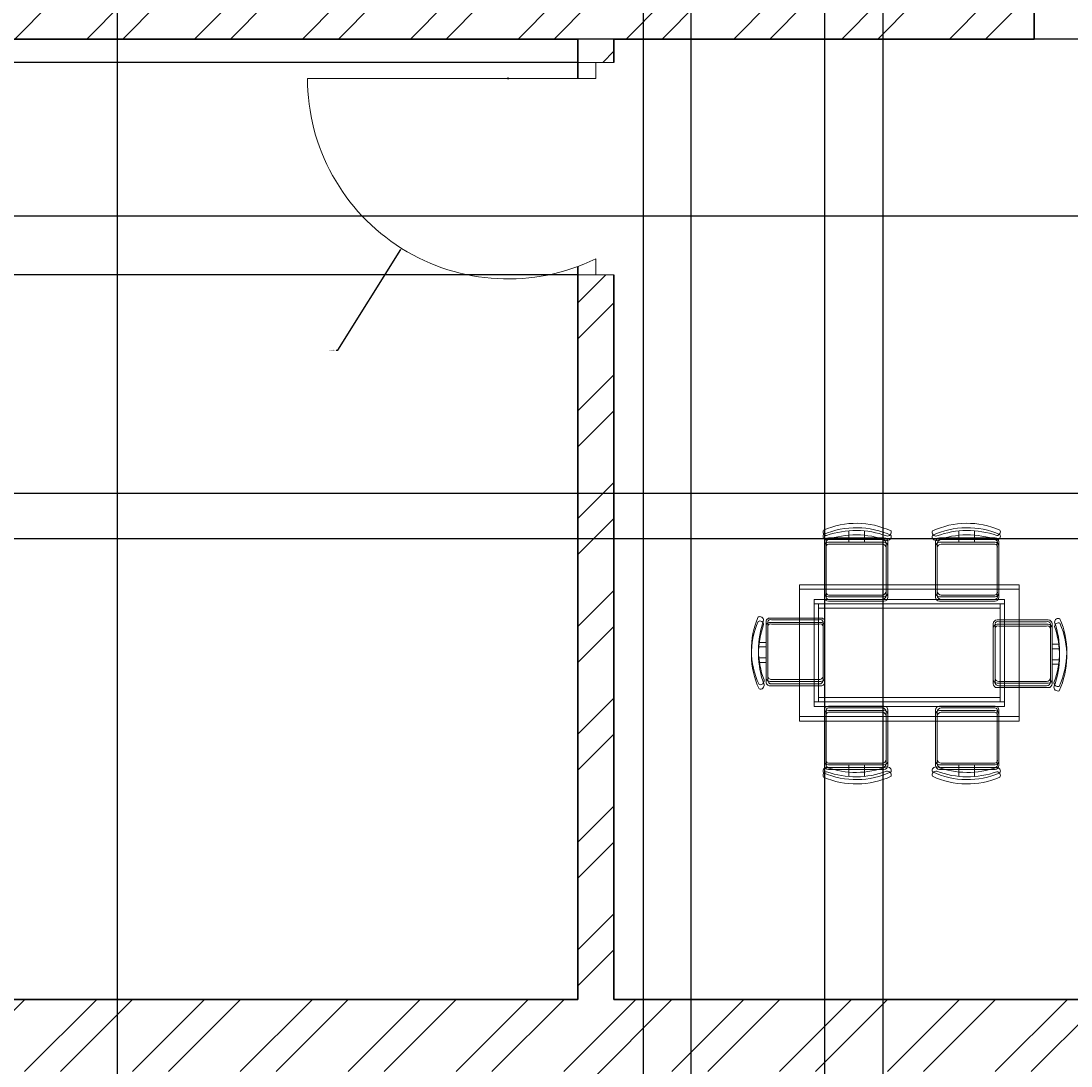
# Model space of a CAD drawing. Units: inches. Extents: x 1748 to 2382, y 1346 to 2284.
# Tile 21 of 26: x 1956 to 2088, y 1971 to 2102. Entities that reach past the tile are written whole.
import ezdxf

# ---------------------------------------------------------------- set-up
doc = ezdxf.new("R2010")
doc.units = ezdxf.units.IN
for name, color, linetype, lineweight in [('A-ANNO-DIMS', 2, 'Continuous', 18), ('A-DOOR', 21, 'Continuous', 18), ('A-FURN', 8, 'Continuous', 13), ('A-WALL', 7, 'Continuous', 35), ('A-WALL-PATT', 9, 'Continuous', 13)]:
    doc.layers.add(name, color=color, linetype=linetype, lineweight=lineweight)
doc.styles.get("Standard").update_dxf_attribs({"font": 'arial.ttf'})
doc.dimstyles.get("Standard").update_dxf_attribs({"dimtxt": 0.18, "dimasz": 0.18, "dimexe": 0.18, "dimexo": 0.0625, "dimgap": 0.09, "dimtad": 0, "dimtih": 1, "dimtoh": 1, "dimdec": 4, "dimzin": 0, "dimdsep": 46, "dimtxsty": 'Standard', "dimcen": 0.09, "dimadec": 0, "dimazin": 0, "dimtfac": 1, "dimtdec": 4, "dimtofl": 0, "dimtmove": 0, "dimatfit": 3, "dimfxl": 1, "dimtolj": 1, "dimtzin": 0, "dimarcsym": 0})

# ---------------------------------------------------------------- blocks, each defined once
blk = doc.blocks.new('TABLE-DINING')
for points in [[(0, 17.02), (27.45, 17.02), (27.45, 0.55), (0, 0.55)], [(0, 17.02), (27.45, 17.02), (27.45, 0.55), (0, 0.55)], [(0, 16.47), (27.45, 16.47), (27.45, 0), (0, 0)], [(0, 16.47), (27.45, 16.47), (27.45, 0), (0, 0)], [(1.83, 15.19), (25.62, 15.19), (25.62, 2.38), (1.83, 2.38)], [(1.83, 15.19), (25.62, 15.19), (25.62, 2.38), (1.83, 2.38)], [(1.83, 14.64), (25.62, 14.64), (25.62, 1.83), (1.83, 1.83)], [(1.83, 14.64), (25.62, 14.64), (25.62, 1.83), (1.83, 1.83)], [(2.38, 14.64), (25.07, 14.64), (25.07, 2.93), (2.38, 2.93)], [(2.38, 14.64), (25.07, 14.64), (25.07, 2.93), (2.38, 2.93)], [(2.38, 14.09), (25.07, 14.09), (25.07, 2.38), (2.38, 2.38)], [(2.38, 14.09), (25.07, 14.09), (25.07, 2.38), (2.38, 2.38)]]:
    blk.add_lwpolyline(points, close=True)
blk = doc.blocks.new('CHAIR-DINING-END')
for points in [[(7.35, 8.4, 0.414214), (6.87, 8.88), (0.49, 8.88, 0.414214), (0, 8.4), (0, 1.46, 0.414214), (0.49, 0.97), (6.87, 0.97, 0.414214), (7.35, 1.46), (7.35, 8.4)], [(7.35, 8.4, 0.414214), (6.87, 8.88), (0.49, 8.88, 0.414214), (0, 8.4), (0, 1.46, 0.414214), (0.49, 0.97), (6.87, 0.97, 0.414214), (7.35, 1.46), (7.35, 8.4)], [(7.35, 7.85, 0.414214), (6.87, 8.33), (0.49, 8.33, 0.414214), (0, 7.85), (0, 0.91, 0.414214), (0.49, 0.42), (6.87, 0.42, 0.414214), (7.35, 0.91), (7.35, 7.85)], [(7.35, 7.85, 0.414214), (6.87, 8.33), (0.49, 8.33, 0.414214), (0, 7.85), (0, 0.91, 0.414214), (0.49, 0.42), (6.87, 0.42, 0.414214), (7.35, 0.91), (7.35, 7.85)], [(7.65, 8.61, -0.175809), (7.6, 1.14, 0.578392), (8.22, 0.57, 0.214524), (8.33, 9.01, 0.552014), (7.65, 8.61, -0.065079)], [(7.65, 8.61, -0.175809), (7.6, 1.14, 0.578392), (8.22, 0.57, 0.214524), (8.33, 9.01, 0.552014), (7.65, 8.61, -0.065079)], [(7.65, 8.06, -0.175809), (7.6, 0.59, 0.578392), (8.22, 0.02, 0.214524), (8.33, 8.46, 0.552014), (7.65, 8.06, -0.065079)], [(7.65, 8.06, -0.175809), (7.6, 0.59, 0.578392), (8.22, 0.02, 0.214524), (8.33, 8.46, 0.552014), (7.65, 8.06, -0.065079)], [(7.35, 3.89), (8.23, 3.89, -0.064759)], [(7.35, 3.89), (8.23, 3.89, -0.064759)], [(7.35, 3.34), (8.23, 3.34, -0.064759)], [(7.35, 3.34), (8.23, 3.34, -0.064759)]]:
    blk.add_lwpolyline(points, format="xyb")
for points in [[(7.13, 8.39), (7.13, 1.67, -0.414214), (6.65, 1.19), (0.7, 1.19, -0.414214), (0.22, 1.67), (0.22, 8.39, -0.512069), (0.7, 8.66), (6.65, 8.66, -0.512069)], [(7.13, 8.39), (7.13, 1.67, -0.414214), (6.65, 1.19), (0.7, 1.19, -0.414214), (0.22, 1.67), (0.22, 8.39, -0.512069), (0.7, 8.66), (6.65, 8.66, -0.512069)], [(7.13, 7.84), (7.13, 1.13, -0.414214), (6.65, 0.64), (0.7, 0.64, -0.414214), (0.22, 1.13), (0.22, 7.84, -0.512069), (0.7, 8.11), (6.65, 8.11, -0.512069)], [(7.13, 7.84), (7.13, 1.12, -0.414214), (6.65, 0.64), (0.7, 0.64, -0.414214), (0.22, 1.12), (0.22, 7.84, -0.512069), (0.7, 8.11), (6.65, 8.11, -0.512069)]]:
    blk.add_lwpolyline(points, format="xyb", close=True)
for points in [[(8.25, 5.84), (7.35, 5.84)], [(8.25, 5.84), (7.35, 5.84)], [(8.25, 5.29), (7.35, 5.29)], [(8.25, 5.29), (7.35, 5.29)]]:
    blk.add_lwpolyline(points)
blk = doc.blocks.new('*D51')
at = {"layer": 'A-ANNO-DIMS', "color": 0, "lineweight": -2, "transparency": 16777216}
for p, q in [((1968.44, 2223.79), (1968.44, 1360.47)), ((2040.07, 2223.79), (2040.07, 1360.47)), ((1968.62, 1360.65), (2003.86, 1360.65)), ((2039.89, 1360.65), (2004.65, 1360.65))]:
    blk.add_line(p, q, dxfattribs=at)
at = {"layer": 'A-ANNO-DIMS', "color": 0, "transparency": 16777216}
for points in [[(1968.62, 1360.68), (1968.62, 1360.62), (1968.44, 1360.65)], [(2039.89, 1360.68), (2039.89, 1360.62), (2040.07, 1360.65)]]:
    blk.add_solid(points, dxfattribs=at)
at = {"layer": 'Defpoints', "color": 0, "transparency": 16777216}
for p in [(1968.44, 2223.85), (2040.07, 2223.85), (2040.07, 1360.65)]:
    blk.add_point(p, dxfattribs=at)
at = {"layer": 'A-ANNO-DIMS', "color": 0, "transparency": 16777216, "insert": (2004.26, 1360.65), "char_height": 0.18, "attachment_point": 5}
blk.add_mtext('\\A1;71.62', dxfattribs=at)
blk = doc.blocks.new('*D52')
at = {"layer": 'A-ANNO-DIMS', "color": 0, "lineweight": -2, "transparency": 16777216}
for p, q in [((2064.07, 2223.79), (2064.07, 1360.47)), ((2091.4, 2223.79), (2091.4, 1360.47)), ((2064.25, 1360.65), (2077.34, 1360.65)), ((2091.22, 1360.65), (2078.13, 1360.65))]:
    blk.add_line(p, q, dxfattribs=at)
at = {"layer": 'A-ANNO-DIMS', "color": 0, "transparency": 16777216}
for points in [[(2064.25, 1360.68), (2064.25, 1360.62), (2064.07, 1360.65)], [(2091.22, 1360.68), (2091.22, 1360.62), (2091.4, 1360.65)]]:
    blk.add_solid(points, dxfattribs=at)
at = {"layer": 'Defpoints', "color": 0, "transparency": 16777216}
for p in [(2064.07, 2223.85), (2091.4, 2223.85), (2091.4, 1360.65)]:
    blk.add_point(p, dxfattribs=at)
at = {"layer": 'A-ANNO-DIMS', "color": 0, "transparency": 16777216, "insert": (2077.73, 1360.65), "char_height": 0.18, "attachment_point": 5}
blk.add_mtext('\\A1;27.33', dxfattribs=at)
blk = doc.blocks.new('*D57')
at = {"layer": 'A-ANNO-DIMS', "color": 0, "lineweight": -2, "transparency": 16777216}
for p, q in [((2288.4, 2099.35), (1779.88, 2099.35)), ((1780.06, 2099.17), (1780.06, 2088.46)), ((1780.06, 2077.38), (1780.06, 2088.09)), ((2288.4, 2077.2), (1779.88, 2077.2))]:
    blk.add_line(p, q, dxfattribs=at)
at = {"layer": 'A-ANNO-DIMS', "color": 0, "transparency": 16777216}
for points in [[(1780.03, 2099.17), (1780.09, 2099.17), (1780.06, 2099.35)], [(1780.03, 2077.38), (1780.09, 2077.38), (1780.06, 2077.2)]]:
    blk.add_solid(points, dxfattribs=at)
at = {"layer": 'Defpoints', "color": 0, "transparency": 16777216}
for p in [(1780.06, 2099.35), (2288.46, 2099.35), (2288.46, 2077.2)]:
    blk.add_point(p, dxfattribs=at)
at = {"layer": 'A-ANNO-DIMS', "color": 0, "transparency": 16777216, "insert": (1780.06, 2088.28), "char_height": 0.18, "attachment_point": 5}
blk.add_mtext('\\A1;22.15', dxfattribs=at)
blk = doc.blocks.new('*D63')
at = {"layer": 'A-ANNO-DIMS', "color": 0, "lineweight": -2, "transparency": 16777216}
for p, q in [((2253.72, 2042.57), (1779.88, 2042.57)), ((1780.06, 2042.39), (1780.06, 2039.92)), ((1780.06, 2037.08), (1780.06, 2039.55)), ((2253.72, 2036.9), (1779.88, 2036.9))]:
    blk.add_line(p, q, dxfattribs=at)
at = {"layer": 'A-ANNO-DIMS', "color": 0, "transparency": 16777216}
for points in [[(1780.03, 2042.39), (1780.09, 2042.39), (1780.06, 2042.57)], [(1780.03, 2037.08), (1780.09, 2037.08), (1780.06, 2036.9)]]:
    blk.add_solid(points, dxfattribs=at)
at = {"layer": 'Defpoints', "color": 0, "transparency": 16777216}
for p in [(1780.06, 2042.57), (2253.78, 2042.57), (2253.78, 2036.9)]:
    blk.add_point(p, dxfattribs=at)
at = {"layer": 'A-ANNO-DIMS', "color": 0, "transparency": 16777216, "insert": (1780.06, 2039.74), "char_height": 0.18, "attachment_point": 5}
blk.add_mtext('\\A1;5.673', dxfattribs=at)
blk = doc.blocks.new('*D76')
at = {"layer": 'A-ANNO-DIMS', "color": 0, "lineweight": -2, "transparency": 16777216}
for p, q in [((2025.9, 2096.43), (1779.88, 2096.43)), ((1780.06, 2096.25), (1780.06, 2083.35)), ((1780.06, 2070.08), (1780.06, 2082.98)), ((2025.9, 2069.9), (1779.88, 2069.9))]:
    blk.add_line(p, q, dxfattribs=at)
at = {"layer": 'A-ANNO-DIMS', "color": 0, "transparency": 16777216}
for points in [[(1780.03, 2096.25), (1780.09, 2096.25), (1780.06, 2096.43)], [(1780.03, 2070.08), (1780.09, 2070.08), (1780.06, 2069.9)]]:
    blk.add_solid(points, dxfattribs=at)
at = {"layer": 'Defpoints', "color": 0, "transparency": 16777216}
for p in [(1780.06, 2096.43), (2025.96, 2096.43), (2025.96, 2069.9)]:
    blk.add_point(p, dxfattribs=at)
at = {"layer": 'A-ANNO-DIMS', "color": 0, "transparency": 16777216, "insert": (1780.06, 2083.16), "char_height": 0.18, "attachment_point": 5}
blk.add_mtext('\\A1;26.535', dxfattribs=at)
blk = doc.blocks.new('*D78')
at = {"layer": 'A-ANNO-DIMS', "color": 0, "lineweight": -2, "transparency": 16777216}
for p, q in [((2034.13, 2132.54), (2034.13, 1360.47)), ((2056.8, 2127.06), (2056.8, 1360.47)), ((2034.31, 1360.65), (2045, 1360.65)), ((2056.62, 1360.65), (2045.93, 1360.65))]:
    blk.add_line(p, q, dxfattribs=at)
at = {"layer": 'A-ANNO-DIMS', "color": 0, "transparency": 16777216}
for points in [[(2034.31, 1360.68), (2034.31, 1360.62), (2034.13, 1360.65)], [(2056.62, 1360.68), (2056.62, 1360.62), (2056.8, 1360.65)]]:
    blk.add_solid(points, dxfattribs=at)
at = {"layer": 'Defpoints', "color": 0, "transparency": 16777216}
for p in [(2034.13, 2132.6), (2056.8, 2127.13), (2056.8, 1360.65)]:
    blk.add_point(p, dxfattribs=at)
at = {"layer": 'A-ANNO-DIMS', "color": 0, "transparency": 16777216, "insert": (2045.47, 1360.65), "char_height": 0.18, "attachment_point": 5}
blk.add_mtext('\\A1;22.663', dxfattribs=at)
blk = doc.blocks.new('*D87')
at = {"layer": 'A-ANNO-DIMS', "color": 0, "lineweight": -2, "transparency": 16777216}
for p, q in [((2017.17, 2094.43), (2017.35, 2094.43)), ((2017.26, 2094.34), (2017.26, 2094.52)), ((1995.99, 2060.46), (2003.88, 2073.04)), ((1995.81, 2060.46), (1995.99, 2060.46))]:
    blk.add_line(p, q, dxfattribs=at)
at = {"layer": 'A-ANNO-DIMS', "color": 0, "transparency": 16777216}
blk.add_solid([(2003.85, 2073.06), (2003.9, 2073.03), (2003.97, 2073.2)], dxfattribs=at)
at = {"layer": 'Defpoints', "color": 0, "transparency": 16777216}
for p in [(2017.26, 2094.43), (2003.97, 2073.2)]:
    blk.add_point(p, dxfattribs=at)
at = {"layer": 'A-ANNO-DIMS', "color": 0, "transparency": 16777216, "insert": (1995.27, 2060.46), "char_height": 0.18, "attachment_point": 5}
blk.add_mtext('\\A1;R25.053', dxfattribs=at)

msp = doc.modelspace()

# ---------------------------------------------------------------- hatches: boundary and pattern name
at = {"layer": 'A-WALL-PATT'}
h = msp.add_hatch(dxfattribs=at)
h.set_pattern_fill('ANSI32', color=256)
h.paths.add_polyline_path([(1908.4445, 2232.8497), (1821.9607, 2232.8497), (1821.9607, 2223.8497), (1865.4607, 2223.8497), (1865.4607, 2209.9185), (1869.9607, 2209.9185), (1869.9607, 2223.8497), (1908.4445, 2223.8497), (1908.4445, 2228.3497)])
h.paths.add_polyline_path([(2040.0683, 2232.8497), (1968.4445, 2232.8497), (1968.4445, 2223.8497), (2025.9607, 2223.8497), (2025.9607, 2130.3497), (2032.1341, 2130.3497), (2032.1341, 2132.5997), (2032.1341, 2134.8497), (2030.4607, 2134.8497), (2030.4607, 2223.8497), (2040.0683, 2223.8497)])
h.paths.add_polyline_path([(2091.3969, 2232.8497), (2064.0683, 2232.8497), (2064.0683, 2223.8497), (2078.4607, 2223.8497), (2078.4607, 2134.8497), (2051.1563, 2134.8497), (2051.1563, 2130.3497), (2078.4607, 2130.3497), (2078.4607, 2128.6813), (2082.9607, 2128.6813), (2082.9607, 2130.3497), (2086.1879, 2130.3497), (2086.1879, 2132.5997), (2086.1879, 2134.8497), (2082.9607, 2134.8497), (2082.9607, 2223.8497), (2091.3969, 2223.8497), (2091.3969, 2228.3497)])
h.paths.add_polyline_path([(2167.0164, 2232.8497), (2115.3969, 2232.8497), (2115.3969, 2223.8497), (2130.9607, 2223.8497), (2130.9607, 2134.8497), (2106.9607, 2134.8497), (2106.9607, 2130.3497), (2135.4607, 2130.3497), (2135.4607, 2223.8497), (2167.0164, 2223.8497), (2167.0164, 2228.3497)])
h.paths.add_polyline_path([(1869.9607, 2149.9185), (1865.4607, 2149.9185), (1865.4607, 2127.8942), (1869.9607, 2127.8942)])
h.paths.add_polyline_path([(2082.9607, 2104.4871), (2080.7107, 2104.4871), (2078.4607, 2104.4871), (2078.4607, 2103.8497), (1869.9607, 2103.8497), (1869.9607, 2108.6062), (1867.7107, 2108.6062), (1865.4607, 2108.6062), (1865.4607, 2103.8497), (1821.9607, 2103.8497), (1821.9607, 2099.3497), (1865.4607, 2099.3497), (1865.4607, 2094.7509), (1869.9607, 2094.7509), (1869.9607, 2099.3497), (2025.9607, 2099.3497), (2025.9607, 2096.4326), (2030.4607, 2096.4326), (2030.4607, 2099.3497), (2082.9607, 2099.3497)])
h.paths.add_polyline_path([(1928.9457, 1401.1212), (2176.8693, 1401.1212), (2176.8693, 1438.214), (1928.9457, 1438.214)], flags=9)
h.paths.add_polyline_path([(2122.2668, 2048.1927), (2177.9387, 2048.1927), (2177.9387, 2066.85), (2122.2668, 2066.85)], flags=9)
h.paths.add_polyline_path([(2272.688, 2153.8197), (2272.688, 2216.746), (2262.3845, 2216.746), (2262.3845, 2153.8197)], flags=9)
h.paths.add_polyline_path([(2157.2928, 2166.5593), (2196.3822, 2166.5593), (2196.3822, 2185.2167), (2157.2928, 2185.2167)], flags=9)
h.paths.add_polyline_path([(2089.3407, 2162.0698), (2124.3987, 2162.0698), (2124.3987, 2180.7272), (2089.3407, 2180.7272)], flags=9)
h.paths.add_polyline_path([(2037.4521, 2160.0913), (2072.5101, 2160.0913), (2072.5101, 2178.7486), (2037.4521, 2178.7486)], flags=9)
h.paths.add_polyline_path([(1884.7894, 2104.1554), (1923.6297, 2104.1554), (1923.6297, 2122.8127), (1884.7894, 2122.8127)], flags=9)
h.paths.add_polyline_path([(1851.2832, 2142.9749), (1851.2832, 2199.3051), (1840.9796, 2199.3051), (1840.9796, 2142.9749)], flags=9)
h.paths.add_polyline_path([(1844.8763, 2017.2834), (1844.8763, 2073.6136), (1834.5728, 2073.6136), (1834.5728, 2017.2834)], flags=9)
h.paths.add_polyline_path([(1897.1577, 2073.1279), (1935.9981, 2073.1279), (1935.9981, 2091.7853), (1897.1577, 2091.7853)], flags=9)
h.paths.add_polyline_path([(1952.3395, 1802.4231), (2008.0114, 1802.4231), (2008.0114, 1821.0805), (1952.3395, 1821.0805)], flags=9)
h.paths.add_polyline_path([(1978.8184, 1857.6841), (2017.7338, 1857.6841), (2017.7338, 1876.3415), (1978.8184, 1876.3415)], flags=9)
h.paths.add_polyline_path([(1979.6513, 1925.9516), (2008.8089, 1925.9516), (2008.8089, 1944.6089), (1979.6513, 1944.6089)], flags=9)
h.paths.add_polyline_path([(1838.5553, 1860.3527), (1877.3957, 1860.3527), (1877.3957, 1879.01), (1838.5553, 1879.01)], flags=9)
h.paths.add_polyline_path([(1883.9018, 1787.3013), (1883.9018, 1843.6315), (1873.5983, 1843.6315), (1873.5983, 1787.3013)], flags=9)
h.paths.add_polyline_path([(1873.7079, 1509.1938), (1873.7079, 1583.7709), (1863.4044, 1583.7709), (1863.4044, 1509.1938)], flags=9)
h.paths.add_polyline_path([(1916.2259, 1603.3681), (1955.0663, 1603.3681), (1955.0663, 1622.0254), (1916.2259, 1622.0254)], flags=9)
h.paths.add_polyline_path([(1876.3013, 1636.757), (1876.3013, 1693.0871), (1865.9978, 1693.0871), (1865.9978, 1636.757)], flags=9)
h.paths.add_polyline_path([(1921.3138, 1521.8316), (1964.0662, 1521.8316), (1964.0662, 1540.489), (1921.3138, 1540.489)], flags=9)
h.paths.add_polyline_path([(2017.5657, 1497.5078), (2046.7983, 1497.5078), (2046.7983, 1516.1651), (2017.5657, 1516.1651)], flags=9)
h.paths.add_polyline_path([(2066.8661, 1499.3902), (2096.0988, 1499.3902), (2096.0988, 1518.0475), (2066.8661, 1518.0475)], flags=9)
h.paths.add_polyline_path([(2155.4835, 1571.6596), (2198.2358, 1571.6596), (2198.2358, 1590.3169), (2155.4835, 1590.3169)], flags=9)
h.paths.add_polyline_path([(2094.9136, 1664.6812), (2150.5855, 1664.6812), (2150.5855, 1683.3386), (2094.9136, 1683.3386)], flags=9)
h.paths.add_polyline_path([(2257.6902, 1863.1628), (2269.8935, 1863.1628), (2269.8935, 1873.4664), (2257.6902, 1873.4664)], flags=9)
h.paths.add_polyline_path([(2164.0748, 1880.3089), (2189.8694, 1880.3089), (2189.8694, 1890.6124), (2164.0748, 1890.6124)], flags=9)
h.paths.add_polyline_path([(2239.4394, 1931.0585), (2268.8187, 1931.0585), (2268.8187, 1949.7159), (2239.4394, 1949.7159)], flags=9)
h = msp.add_hatch(dxfattribs=at)
h.set_pattern_fill('ANSI32', color=256)
h.paths.add_polyline_path([(1900.6426, 1652.723), (1896.1426, 1652.723), (1896.1426, 1629.9029), (1900.6426, 1629.9029)])
h.paths.add_polyline_path([(2206.0699, 1859.3497), (2197.0699, 1859.3497), (2197.0699, 1734.8497), (2206.0699, 1734.8497)], flags=17)
h.paths.add_polyline_path([(2297.4607, 1865.3269), (2288.4607, 1865.3269), (2288.4607, 1734.8497), (2206.0699, 1734.8497), (2180.4551, 1734.8497), (2180.4551, 1725.8497), (2197.0699, 1725.8497), (2206.0699, 1725.8497), (2288.4607, 1725.8497), (2288.4607, 1705.3038), (2297.4607, 1705.3038)])
h.paths.add_polyline_path([(2139.9607, 1815.8001), (2135.4607, 1815.8001), (2130.9607, 1815.8001), (2130.9607, 1734.8497), (1900.6426, 1734.8497), (1900.6426, 1738.9477), (1898.3926, 1738.9477), (1896.1426, 1738.9477), (1896.1426, 1734.8497), (1857.1426, 1734.8497), (1857.1426, 1725.8497), (1896.1426, 1725.8497), (1896.1426, 1712.723), (1900.6426, 1712.723), (1900.6426, 1725.8497), (2006.4607, 1725.8497), (2006.4607, 1637.448), (2010.9607, 1637.448), (2010.9607, 1725.8497), (2139.9607, 1725.8497), (2147.389, 1725.8497), (2147.389, 1730.3497), (2147.389, 1734.8497), (2139.9607, 1734.8497)])
h.paths.add_polyline_path([(2149.8497, 1917.8497), (2149.8497, 1922.3497), (2139.9607, 1922.3497), (2139.9607, 1979.3497), (2030.4607, 1979.3497), (2030.4607, 2069.8971), (2028.2107, 2069.8971), (2025.9607, 2069.8971), (2025.9607, 1979.3497), (1869.9607, 1979.3497), (1869.9607, 1998.93), (1865.4607, 1998.93), (1865.4607, 1979.3497), (1821.9607, 1979.3497), (1821.9607, 1952.7922), (1826.9306, 1952.7922), (1830.9607, 1952.7922), (1830.9607, 1970.3497), (1962.9607, 1970.3497), (1962.9607, 1926.5713), (1967.4607, 1926.5713), (1967.4607, 1970.3497), (2027.4607, 1970.3497), (2027.4607, 1898.3497), (2004.9604, 1898.3497), (2004.9604, 1893.8497), (2027.4607, 1893.8497), (2027.4607, 1859.3497), (1958.8973, 1859.3497), (1958.8973, 1854.8497), (2047.917, 1854.8497), (2047.917, 1859.3497), (2031.9607, 1859.3497), (2031.9607, 1970.3497), (2130.9607, 1970.3497), (2130.9607, 1859.3497), (2104.9565, 1859.3497), (2104.9565, 1854.8497), (2130.9607, 1854.8497), (2130.9607, 1849.0684), (2139.9607, 1849.0684), (2139.9607, 1913.3497), (2149.8497, 1913.3497)])
h.paths.add_polyline_path([(1928.9996, 1859.3497), (1830.9607, 1859.3497), (1830.9607, 1892.7922), (1821.9607, 1892.7922), (1821.9607, 1854.8497), (1896.1426, 1854.8497), (1896.1426, 1836.6443), (1898.378, 1836.6443), (1900.6426, 1836.6443), (1900.6426, 1854.8497), (1928.9996, 1854.8497), (1928.9996, 1857.0997)])
h.paths.add_polyline_path([(1980.9604, 1896.0997), (1980.9604, 1898.3497), (1967.4607, 1898.3497), (1967.4607, 1902.3846), (1962.9607, 1902.3846), (1962.9607, 1859.3497), (1967.4607, 1859.3497), (1967.4607, 1893.8497), (1980.9604, 1893.8497)], flags=17)
h.paths.add_polyline_path([(1900.6426, 1776.6443), (1896.1426, 1776.6443), (1896.1426, 1758.0891), (1900.6426, 1758.0891)], flags=17)
h.paths.add_polyline_path([(2297.4607, 2017.2008), (2288.4607, 2017.2008), (2288.4607, 1979.3497), (2213.4607, 1979.3497), (2213.4607, 1922.3497), (2183.3516, 1922.3497), (2183.3516, 1913.3497), (2213.4607, 1913.3497), (2236.234, 1913.3497), (2236.234, 1922.3497), (2222.4607, 1922.3497), (2222.4607, 1931.3497), (2222.4607, 1970.3497), (2288.4607, 1970.3497), (2288.4607, 1922.3497), (2272.1921, 1922.3497), (2272.1921, 1913.3497), (2288.4607, 1913.3497), (2288.4607, 1901.3269), (2297.4607, 1901.3269)])

# ---------------------------------------------------------------- linework, layer by layer
at = {"layer": 'A-DOOR'}
for p, q in [((2025.9607, 2096.4326), (2030.4607, 2096.4326)), ((2030.4607, 2096.4326), (2028.2107, 2096.4326)), ((2028.2107, 2096.4326), (2028.2107, 2094.4326)), ((2028.2107, 2094.4326), (1992.2107, 2094.4326)), ((2028.2107, 2069.8971), (2028.2107, 2071.8971)), ((2025.9607, 2069.8971), (2030.4607, 2069.8971)), ((2030.4607, 2069.8971), (2028.2107, 2069.8971))]:
    msp.add_line(p, q, dxfattribs=at)
msp.add_arc((2017.2641, 2094.4326), 25.0534, 180, 295.908118, dxfattribs=at)
at = {"layer": 'A-FURN'}
for points in [[(2057.0522, 2037.3215, -0.17580919), (2064.5276, 2037.2649, 0.57839206), (2065.0939, 2037.8876, 0.21452438), (2056.6557, 2038.0008, 0.55201397), (2057.0522, 2037.3215, -0.06507904)], [(2057.0522, 2037.3212, -0.17580919), (2064.5276, 2037.2646, 0.57839206), (2065.0939, 2037.8873, 0.21452438), (2056.6558, 2038.0005, 0.55201397), (2057.0522, 2037.3212, -0.06507904)], [(2057.0522, 2036.7726, -0.17580919), (2064.5276, 2036.716, 0.57839206), (2065.0939, 2037.3387, 0.21452438), (2056.6557, 2037.4519, 0.55201397), (2057.0522, 2036.7726, -0.06507904)], [(2057.0522, 2036.7723, -0.17580919), (2064.5276, 2036.7157, 0.57839206), (2065.0939, 2037.3384, 0.21452438), (2056.6558, 2037.4516, 0.55201397), (2057.0522, 2036.7723, -0.06507904)], [(2070.821, 2037.2649, -0.57839206), (2070.2546, 2037.8876, -0.21452438), (2078.6928, 2038.0008, -0.55201397), (2078.2964, 2037.3215, 0.1758092), (2070.821, 2037.2649)], [(2070.821, 2037.2646, -0.57839206), (2070.2547, 2037.8873, -0.21452438), (2078.6928, 2038.0005, -0.55201397), (2078.2964, 2037.3212, 0.1758092), (2070.821, 2037.2646)], [(2070.821, 2036.716, -0.57839206), (2070.2546, 2037.3387, -0.21452438), (2078.6928, 2037.4519, -0.55201397), (2078.2964, 2036.7726, 0.1758092), (2070.821, 2036.716)], [(2070.821, 2036.7157, -0.57839206), (2070.2547, 2037.3384, -0.21452438), (2078.6928, 2037.4516, -0.55201397), (2078.2964, 2036.7723, 0.1758092), (2070.821, 2036.7157)], [(2064.2105, 2037.0215), (2057.2705, 2037.0215, 0.41421356), (2056.785, 2036.536), (2056.785, 2030.1548, 0.41421356), (2057.2705, 2029.6693), (2064.2105, 2029.6693, 0.41421356), (2064.696, 2030.1548), (2064.696, 2036.536, 0.41421356), (2064.2105, 2037.0215)], [(2064.2105, 2037.0212), (2057.2705, 2037.0212, 0.41421356), (2056.785, 2036.5357), (2056.785, 2030.1545, 0.41421356), (2057.2705, 2029.669), (2064.2105, 2029.669, 0.41421356), (2064.696, 2030.1545), (2064.696, 2036.5357, 0.41421356), (2064.2105, 2037.0212)], [(2061.7728, 2037.0215), (2061.7728, 2037.8992, -0.06475861)], [(2061.7728, 2037.0212), (2061.7728, 2037.8989, -0.06475861)], [(2061.7728, 2036.4726), (2061.7728, 2037.3503, -0.06475861)], [(2061.7728, 2036.4723), (2061.7728, 2037.35, -0.06475861)], [(2078.0781, 2037.0215, -0.41421356), (2078.5636, 2036.536), (2078.5636, 2030.1548, -0.41421356), (2078.0781, 2029.6693), (2071.1381, 2029.6693, -0.41421356), (2070.6526, 2030.1548), (2070.6526, 2036.536, -0.41421356), (2071.1381, 2037.0215), (2078.0781, 2037.0215)], [(2078.0781, 2037.0212, -0.41421356), (2078.5636, 2036.5357), (2078.5636, 2030.1545, -0.41421356), (2078.0781, 2029.669), (2071.1381, 2029.669, -0.41421356), (2070.6526, 2030.1545), (2070.6526, 2036.5357, -0.41421356), (2071.1381, 2037.0212), (2078.0781, 2037.0212)], [(2073.5758, 2037.0215), (2073.5758, 2037.8992, 0.06475861)], [(2073.5758, 2037.0212), (2073.5758, 2037.8989, 0.06475861)], [(2073.5758, 2036.4726), (2073.5758, 2037.3503, 0.06475861)], [(2073.5758, 2036.4723), (2073.5758, 2037.35, 0.06475861)], [(2064.2105, 2036.4726), (2057.2705, 2036.4726, 0.41421356), (2056.785, 2035.987), (2056.785, 2029.6059, 0.41421356), (2057.2705, 2029.1204), (2064.2105, 2029.1204, 0.41421356), (2064.696, 2029.6059), (2064.696, 2035.987, 0.41421356), (2064.2105, 2036.4726)], [(2064.2105, 2036.4723), (2057.2705, 2036.4723, 0.41421356), (2056.785, 2035.9868), (2056.785, 2029.6056, 0.41421356), (2057.2705, 2029.1201), (2064.2105, 2029.1201, 0.41421356), (2064.696, 2029.6056), (2064.696, 2035.9868, 0.41421356), (2064.2105, 2036.4723)], [(2078.0781, 2036.4726, -0.41421356), (2078.5636, 2035.987), (2078.5636, 2029.6059, -0.41421356), (2078.0781, 2029.1204), (2071.1381, 2029.1204, -0.41421356), (2070.6526, 2029.6059), (2070.6526, 2035.987, -0.41421356), (2071.1381, 2036.4726), (2078.0781, 2036.4726)], [(2078.0781, 2036.4723, -0.41421356), (2078.5636, 2035.9868), (2078.5636, 2029.6056, -0.41421356), (2078.0781, 2029.1201), (2071.1381, 2029.1201, -0.41421356), (2070.6526, 2029.6056), (2070.6526, 2035.9868, -0.41421356), (2071.1381, 2036.4723), (2078.0781, 2036.4723)], [(2085.2123, 2026.2889, 0.41421356), (2084.7268, 2026.7744), (2078.3456, 2026.7744, 0.41421356), (2077.8601, 2026.2889), (2077.8601, 2019.3489, 0.41421356), (2078.3456, 2018.8634), (2084.7268, 2018.8634, 0.41421356), (2085.2123, 2019.3489), (2085.2123, 2026.2889)], [(2085.2123, 2026.2886, 0.41421356), (2084.7268, 2026.7741), (2078.3456, 2026.7741, 0.41421356), (2077.8601, 2026.2886), (2077.8601, 2019.3486, 0.41421356), (2078.3456, 2018.8631), (2084.7268, 2018.8631, 0.41421356), (2085.2123, 2019.3486), (2085.2123, 2026.2886)], [(2085.2123, 2025.74, 0.41421356), (2084.7268, 2026.2255), (2078.3456, 2026.2255, 0.41421356), (2077.8601, 2025.74), (2077.8601, 2018.8, 0.41421356), (2078.3456, 2018.3145), (2084.7268, 2018.3145, 0.41421356), (2085.2123, 2018.8), (2085.2123, 2025.74)], [(2085.2123, 2025.7397, 0.41421356), (2084.7268, 2026.2252), (2078.3456, 2026.2252, 0.41421356), (2077.8601, 2025.7397), (2077.8601, 2018.7997, 0.41421356), (2078.3456, 2018.3142), (2084.7268, 2018.3142, 0.41421356), (2085.2123, 2018.7997), (2085.2123, 2025.7397)], [(2085.5123, 2026.5072, -0.17580919), (2085.4557, 2019.0318, 0.57839206), (2086.0784, 2018.4655, 0.21452438), (2086.1917, 2026.9036, 0.55201397), (2085.5123, 2026.5072, -0.06507904)], [(2085.5123, 2025.9583, -0.17580919), (2085.4557, 2018.4829, 0.57839206), (2086.0784, 2017.9165, 0.21452438), (2086.1917, 2026.3547, 0.55201397), (2085.5123, 2025.9583, -0.06507904)], [(2085.5123, 2026.5069, -0.17580919), (2085.4557, 2019.0315, 0.57839206), (2086.0785, 2018.4652, 0.21452438), (2086.1917, 2026.9034, 0.55201397), (2085.5123, 2026.5069, -0.06507904)], [(2085.5123, 2025.958, -0.17580919), (2085.4557, 2018.4826, 0.57839206), (2086.0785, 2017.9163, 0.21452438), (2086.1917, 2026.3544, 0.55201397), (2085.5123, 2025.958, -0.06507904)], [(2085.2123, 2021.7866), (2086.09, 2021.7866, -0.06475861)], [(2085.2123, 2021.7863), (2086.09, 2021.7863, -0.06475861)], [(2085.2123, 2021.2377), (2086.09, 2021.2377, -0.06475861)], [(2085.2123, 2021.2374), (2086.09, 2021.2374, -0.06475861)], [(2064.2105, 2008.6557), (2057.2705, 2008.6557, -0.41421356), (2056.785, 2009.1413), (2056.785, 2015.5224, -0.41421356), (2057.2705, 2016.0079), (2064.2105, 2016.0079, -0.41421356), (2064.696, 2015.5224), (2064.696, 2009.1413, -0.41421356), (2064.2105, 2008.6557)], [(2064.2105, 2008.6554), (2057.2705, 2008.6554, -0.41421356), (2056.785, 2009.141), (2056.785, 2015.5221, -0.41421356), (2057.2705, 2016.0076), (2064.2105, 2016.0076, -0.41421356), (2064.696, 2015.5221), (2064.696, 2009.141, -0.41421356), (2064.2105, 2008.6554)], [(2078.0781, 2008.6557, 0.41421356), (2078.5636, 2009.1413), (2078.5636, 2015.5224, 0.41421356), (2078.0781, 2016.0079), (2071.1381, 2016.0079, 0.41421356), (2070.6526, 2015.5224), (2070.6526, 2009.1413, 0.41421356), (2071.1381, 2008.6557), (2078.0781, 2008.6557)], [(2078.0781, 2008.6554, 0.41421356), (2078.5636, 2009.141), (2078.5636, 2015.5221, 0.41421356), (2078.0781, 2016.0076), (2071.1381, 2016.0076, 0.41421356), (2070.6526, 2015.5221), (2070.6526, 2009.141, 0.41421356), (2071.1381, 2008.6554), (2078.0781, 2008.6554)], [(2064.2105, 2008.1068), (2057.2705, 2008.1068, -0.41421356), (2056.785, 2008.5923), (2056.785, 2014.9735, -0.41421356), (2057.2705, 2015.459), (2064.2105, 2015.459, -0.41421356), (2064.696, 2014.9735), (2064.696, 2008.5923, -0.41421356), (2064.2105, 2008.1068)], [(2064.2105, 2008.1065), (2057.2705, 2008.1065, -0.41421356), (2056.785, 2008.5921), (2056.785, 2014.9732, -0.41421356), (2057.2705, 2015.4587), (2064.2105, 2015.4587, -0.41421356), (2064.696, 2014.9732), (2064.696, 2008.5921, -0.41421356), (2064.2105, 2008.1065)], [(2078.0781, 2008.1068, 0.41421356), (2078.5636, 2008.5923), (2078.5636, 2014.9735, 0.41421356), (2078.0781, 2015.459), (2071.1381, 2015.459, 0.41421356), (2070.6526, 2014.9735), (2070.6526, 2008.5923, 0.41421356), (2071.1381, 2008.1068), (2078.0781, 2008.1068)], [(2078.0781, 2008.1065, 0.41421356), (2078.5636, 2008.5921), (2078.5636, 2014.9732, 0.41421356), (2078.0781, 2015.4587), (2071.1381, 2015.4587, 0.41421356), (2070.6526, 2014.9732), (2070.6526, 2008.5921, 0.41421356), (2071.1381, 2008.1065), (2078.0781, 2008.1065)], [(2064.5276, 2008.4123, -0.57839206), (2065.0939, 2007.7896, -0.21452438), (2056.6557, 2007.6764, -0.55201397), (2057.0522, 2008.3557, 0.17580929), (2064.5276, 2008.4123)], [(2064.5276, 2008.412, -0.57839206), (2065.0939, 2007.7893, -0.21452438), (2056.6558, 2007.6761, -0.55201397), (2057.0522, 2008.3554, 0.17580929), (2064.5276, 2008.412)], [(2064.5276, 2007.8634, -0.57839206), (2065.0939, 2007.2407, -0.21452438), (2056.6557, 2007.1275, -0.55201397), (2057.0522, 2007.8068, 0.17580929), (2064.5276, 2007.8634)], [(2064.5276, 2007.8631, -0.57839206), (2065.0939, 2007.2404, -0.21452438), (2056.6558, 2007.1272, -0.55201397), (2057.0522, 2007.8065, 0.17580929), (2064.5276, 2007.8631)], [(2061.7728, 2008.6557), (2061.7728, 2007.778, 0.06475861)], [(2061.7728, 2008.6554), (2061.7728, 2007.7778, 0.06475861)], [(2061.7728, 2008.1068), (2061.7728, 2007.2291, 0.06475861)], [(2061.7728, 2008.1065), (2061.7728, 2007.2288, 0.06475861)], [(2078.2964, 2008.3557, -0.17580928), (2070.821, 2008.4123, 0.57839206), (2070.2546, 2007.7896, 0.21452438), (2078.6928, 2007.6764, 0.55201397), (2078.2964, 2008.3557, -0.06507904)], [(2078.2964, 2008.3554, -0.17580928), (2070.821, 2008.412, 0.57839206), (2070.2547, 2007.7893, 0.21452438), (2078.6928, 2007.6761, 0.55201397), (2078.2964, 2008.3554, -0.06507904)], [(2078.2964, 2007.8068, -0.17580928), (2070.821, 2007.8634, 0.57839206), (2070.2546, 2007.2407, 0.21452438), (2078.6928, 2007.1275, 0.55201397), (2078.2964, 2007.8068, -0.06507904)], [(2078.2964, 2007.8065, -0.17580928), (2070.821, 2007.8631, 0.57839206), (2070.2547, 2007.2404, 0.21452438), (2078.6928, 2007.1272, 0.55201397), (2078.2964, 2007.8065, -0.06507904)], [(2073.5758, 2008.6557), (2073.5758, 2007.778, -0.06475861)], [(2073.5758, 2008.6554), (2073.5758, 2007.7778, -0.06475861)], [(2073.5758, 2008.1068), (2073.5758, 2007.2291, -0.06475861)], [(2073.5758, 2008.1065), (2073.5758, 2007.2288, -0.06475861)]]:
    msp.add_lwpolyline(points, format="xyb", dxfattribs=at)
for points in [[(2057.2735, 2036.8027), (2063.9917, 2036.8027, -0.41421356), (2064.4772, 2036.3172), (2064.4772, 2030.3735, -0.41421356), (2063.9917, 2029.888), (2057.2735, 2029.888, -0.51206948), (2057.0037, 2030.3735), (2057.0037, 2036.3172, -0.51206948)], [(2057.2735, 2036.8025), (2063.9917, 2036.8025, -0.41421356), (2064.4773, 2036.3169), (2064.4773, 2030.3733, -0.41421356), (2063.9917, 2029.8877), (2057.2735, 2029.8877, -0.51206948), (2057.0037, 2030.3733), (2057.0037, 2036.3169, -0.51206948)], [(2078.0751, 2036.8027), (2071.3568, 2036.8027, 0.41421356), (2070.8713, 2036.3172), (2070.8713, 2030.3735, 0.41421356), (2071.3568, 2029.888), (2078.0751, 2029.888, 0.51206948), (2078.3448, 2030.3735), (2078.3448, 2036.3172, 0.51206948)], [(2078.0751, 2036.8025), (2071.3569, 2036.8025, 0.41421356), (2070.8713, 2036.3169), (2070.8713, 2030.3733, 0.41421356), (2071.3569, 2029.8877), (2078.0751, 2029.8877, 0.51206948), (2078.3449, 2030.3733), (2078.3449, 2036.3169, 0.51206948)], [(2057.2735, 2036.2538), (2063.9917, 2036.2538, -0.41421356), (2064.4772, 2035.7683), (2064.4772, 2029.8246, -0.41421356), (2063.9917, 2029.3391), (2057.2735, 2029.3391, -0.51206948), (2057.0037, 2029.8246), (2057.0037, 2035.7683, -0.51206948)], [(2057.2735, 2036.2535), (2063.9917, 2036.2535, -0.41421356), (2064.4773, 2035.768), (2064.4773, 2029.8243, -0.41421356), (2063.9917, 2029.3388), (2057.2735, 2029.3388, -0.51206948), (2057.0037, 2029.8243), (2057.0037, 2035.768, -0.51206948)], [(2078.0751, 2036.2538), (2071.3568, 2036.2538, 0.41421356), (2070.8713, 2035.7683), (2070.8713, 2029.8246, 0.41421356), (2071.3568, 2029.3391), (2078.0751, 2029.3391, 0.51206948), (2078.3448, 2029.8246), (2078.3448, 2035.7683, 0.51206948)], [(2078.0751, 2036.2535), (2071.3569, 2036.2535, 0.41421356), (2070.8713, 2035.768), (2070.8713, 2029.8243, 0.41421356), (2071.3569, 2029.3388), (2078.0751, 2029.3388, 0.51206948), (2078.3449, 2029.8243), (2078.3449, 2035.768, 0.51206948)], [(2084.9936, 2026.2859), (2084.9936, 2019.5677, -0.41421356), (2084.508, 2019.0821), (2078.5644, 2019.0821, -0.41421356), (2078.0788, 2019.5677), (2078.0788, 2026.2859, -0.51206948), (2078.5644, 2026.5557), (2084.508, 2026.5557, -0.51206948)], [(2084.9936, 2026.2856), (2084.9936, 2019.5674, -0.41421356), (2084.5081, 2019.0819), (2078.5644, 2019.0819, -0.41421356), (2078.0789, 2019.5674), (2078.0789, 2026.2856, -0.51206948), (2078.5644, 2026.5554), (2084.5081, 2026.5554, -0.51206948)], [(2084.9936, 2025.737), (2084.9936, 2019.0188, -0.41421356), (2084.508, 2018.5332), (2078.5644, 2018.5332, -0.41421356), (2078.0788, 2019.0188), (2078.0788, 2025.737, -0.51206948), (2078.5644, 2026.0068), (2084.508, 2026.0068, -0.51206948)], [(2084.9936, 2025.7367), (2084.9936, 2019.0185, -0.41421356), (2084.5081, 2018.5329), (2078.5644, 2018.5329, -0.41421356), (2078.0789, 2019.0185), (2078.0789, 2025.7367, -0.51206948), (2078.5644, 2026.0065), (2084.5081, 2026.0065, -0.51206948)], [(2057.2735, 2008.8745), (2063.9917, 2008.8745, 0.41421356), (2064.4772, 2009.36), (2064.4772, 2015.3037, 0.41421356), (2063.9917, 2015.7892), (2057.2735, 2015.7892, 0.51206948), (2057.0037, 2015.3037), (2057.0037, 2009.36, 0.51206948)], [(2057.2735, 2008.8742), (2063.9917, 2008.8742, 0.41421356), (2064.4773, 2009.3597), (2064.4773, 2015.3034, 0.41421356), (2063.9917, 2015.7889), (2057.2735, 2015.7889, 0.51206948), (2057.0037, 2015.3034), (2057.0037, 2009.3597, 0.51206948)], [(2078.0751, 2008.8745), (2071.3568, 2008.8745, -0.41421356), (2070.8713, 2009.36), (2070.8713, 2015.3037, -0.41421356), (2071.3568, 2015.7892), (2078.0751, 2015.7892, -0.51206948), (2078.3448, 2015.3037), (2078.3448, 2009.36, -0.51206948)], [(2078.0751, 2008.8742), (2071.3569, 2008.8742, -0.41421356), (2070.8713, 2009.3597), (2070.8713, 2015.3034, -0.41421356), (2071.3569, 2015.7889), (2078.0751, 2015.7889, -0.51206948), (2078.3449, 2015.3034), (2078.3449, 2009.3597, -0.51206948)], [(2057.2735, 2008.3256), (2063.9917, 2008.3256, 0.41421356), (2064.4772, 2008.8111), (2064.4772, 2014.7548, 0.41421356), (2063.9917, 2015.2403), (2057.2735, 2015.2403, 0.51206948), (2057.0037, 2014.7548), (2057.0037, 2008.8111, 0.51206948)], [(2057.2735, 2008.3253), (2063.9917, 2008.3253, 0.41421356), (2064.4773, 2008.8108), (2064.4773, 2014.7545, 0.41421356), (2063.9917, 2015.24), (2057.2735, 2015.24, 0.51206948), (2057.0037, 2014.7545), (2057.0037, 2008.8108, 0.51206948)], [(2078.0751, 2008.3256), (2071.3568, 2008.3256, -0.41421356), (2070.8713, 2008.8111), (2070.8713, 2014.7548, -0.41421356), (2071.3568, 2015.2403), (2078.0751, 2015.2403, -0.51206948), (2078.3448, 2014.7548), (2078.3448, 2008.8111, -0.51206948)], [(2078.0751, 2008.3253), (2071.3569, 2008.3253, -0.41421356), (2070.8713, 2008.8108), (2070.8713, 2014.7545, -0.41421356), (2071.3569, 2015.24), (2078.0751, 2015.24, -0.51206948), (2078.3449, 2014.7545), (2078.3449, 2008.8108, -0.51206948)]]:
    msp.add_lwpolyline(points, format="xyb", close=True, dxfattribs=at)
for points in [[(2059.8302, 2037.9151), (2059.8302, 2037.0215)], [(2059.8302, 2037.9148), (2059.8302, 2037.0212)], [(2059.8302, 2037.3662), (2059.8302, 2036.4726)], [(2059.8302, 2037.3659), (2059.8302, 2036.4723)], [(2075.5184, 2037.9151), (2075.5184, 2037.0215)], [(2075.5184, 2037.9148), (2075.5184, 2037.0212)], [(2075.5184, 2037.3662), (2075.5184, 2036.4726)], [(2075.5184, 2037.3659), (2075.5184, 2036.4723)], [(2086.1059, 2023.7292), (2085.2123, 2023.7292)], [(2086.106, 2023.7289), (2085.2123, 2023.7289)], [(2086.1059, 2023.1803), (2085.2123, 2023.1803)], [(2086.106, 2023.18), (2085.2123, 2023.18)], [(2059.8302, 2007.7621), (2059.8302, 2008.6557)], [(2059.8302, 2007.7618), (2059.8302, 2008.6554)], [(2059.8302, 2007.2132), (2059.8302, 2008.1068)], [(2059.8302, 2007.2129), (2059.8302, 2008.1065)], [(2075.5184, 2007.7621), (2075.5184, 2008.6557)], [(2075.5184, 2007.7618), (2075.5184, 2008.6554)], [(2075.5184, 2007.2132), (2075.5184, 2008.1068)], [(2075.5184, 2007.2129), (2075.5184, 2008.1065)]]:
    msp.add_lwpolyline(points, dxfattribs=at)
at = {"layer": 'A-WALL'}
for p, q in [((2082.9607, 2104.4871), (2082.9607, 2099.3497)), ((1869.9607, 2099.3497), (2025.9607, 2099.3497)), ((2025.9607, 2099.3497), (2025.9607, 2094.4326)), ((2030.4607, 2099.3497), (2030.4607, 2096.4326)), ((2030.4607, 2099.3497), (2082.9607, 2099.3497)), ((2025.9607, 2070.937), (2025.9607, 1979.3497)), ((2030.4607, 2069.8971), (2030.4607, 1979.3497)), ((1869.9607, 1979.3497), (2025.9607, 1979.3497)), ((2030.4607, 1979.3497), (2139.9607, 1979.3497))]:
    msp.add_line(p, q, dxfattribs=at)

# ---------------------------------------------------------------- block references
at = {"layer": 'A-FURN'}
msp.add_blockref('TABLE-DINING', (2053.6579, 2014.1435), dxfattribs=at)
at = {"layer": 'A-FURN', "extrusion": (0, 0, -1), "zscale": -1}
msp.add_blockref('CHAIR-DINING-END', (-2056.8273, 2018.1312), dxfattribs=at)

# ---------------------------------------------------------------- dimensions: what is measured, and where the dimension line sits
at = {"layer": 'A-ANNO-DIMS'}
for base, p1, p2, override, picture, middle in [((2040.0683, 1360.6451), (1968.4445, 2223.8497), (2040.0683, 2223.8497), {"dimdec": 2, "dimlfac": 1, "dimrnd": 0, "dimzin": 0, "dimdsep": 46, "dimlunit": 2}, '*D51', (2004.2564, 1360.6451)), ((2091.3969, 1360.6451), (2064.0683, 2223.8497), (2091.3969, 2223.8497), {"dimdec": 2, "dimlfac": 1, "dimrnd": 0, "dimzin": 0, "dimdsep": 46, "dimlunit": 2}, '*D52', (2077.7326, 1360.6451)), ((2056.7974, 1360.6451), (2034.1341, 2132.5997), (2056.7974, 2127.1257), {"dimdec": 3, "dimlfac": 1, "dimrnd": 0, "dimzin": 0, "dimdsep": 46, "dimlunit": 2}, '*D78', (2045.4658, 1360.6451))]:
    dim = msp.add_linear_dim(base=base, p1=p1, p2=p2, dimstyle='Standard', override=override, dxfattribs=at)
    dim.commit()
    dim.dimension.update_dxf_attribs({"geometry": picture, "text_midpoint": middle})
for base, p1, p2, override, picture, middle in [((1780.0607, 2099.3497), (2288.4607, 2077.2008), (2288.4607, 2099.3497), {"dimdec": 2, "dimlfac": 1, "dimrnd": 0, "dimzin": 0, "dimdsep": 46, "dimlunit": 2}, '*D57', (1780.0607, 2088.2752)), ((1780.06066, 2096.4326), (2025.96066, 2069.89715), (2025.96066, 2096.4326), {"dimdec": 3, "dimlfac": 1, "dimrnd": 0, "dimzin": 0, "dimdsep": 46, "dimlunit": 2}, '*D76', (1780.06066, 2083.16488)), ((1780.0607, 2042.573), (2253.7809, 2036.9), (2253.7809, 2042.573), {"dimdec": 3, "dimlfac": 1, "dimrnd": 0, "dimzin": 0, "dimdsep": 46, "dimlunit": 2}, '*D63', (1780.0607, 2039.7365))]:
    dim = msp.add_linear_dim(base=base, p1=p1, p2=p2, angle=90, dimstyle='Standard', override=override, dxfattribs=at)
    dim.commit()
    dim.dimension.update_dxf_attribs({"geometry": picture, "text_midpoint": middle})
dim = msp.add_radius_dim(center=(2017.2641, 2094.4326), mpoint=(2003.9708, 2073.1967), dimstyle='Standard', override={"dimdec": 3, "dimlfac": 1, "dimrnd": 0, "dimzin": 0, "dimdsep": 46, "dimlunit": 2}, dxfattribs=at)
dim.commit()
dim.dimension.update_dxf_attribs({"geometry": '*D87', "text_midpoint": (1995.2651, 2060.4552), "dimtype": 164})

doc.saveas('drawing.dxf')
